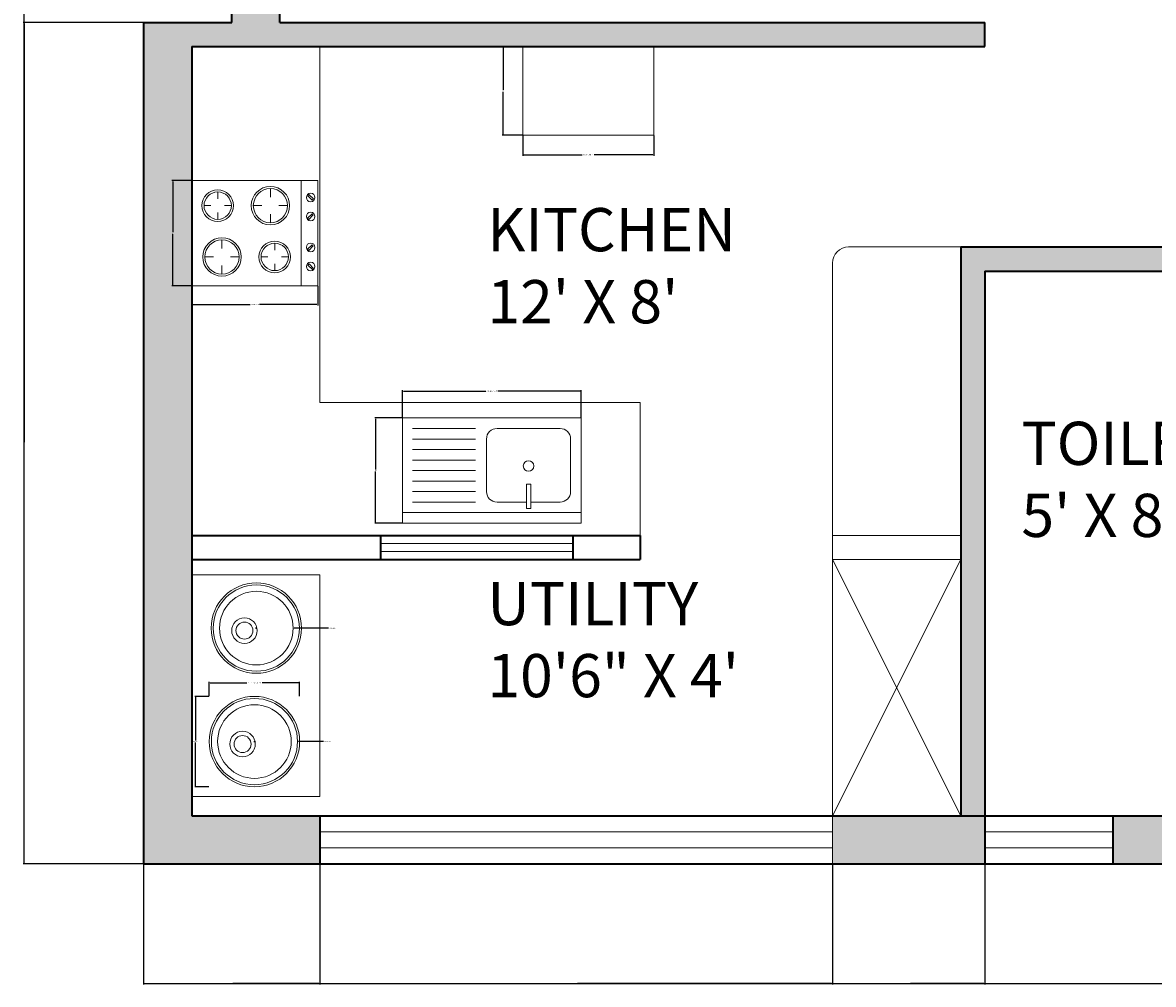
# Model space of a CAD drawing. Units: inches. Extents: x 2 to 2806, y 1095 to 1587.
# Tile 1 of 4: x 2363 to 2575, y 1095 to 1275. Entities that reach past the tile are written whole.
import ezdxf

# ---------------------------------------------------------------- set-up
doc = ezdxf.new("R2010")
doc.units = ezdxf.units.IN
for name, color, linetype, lineweight in [('A-ANNO-DIMS', 2, 'Continuous', 18), ('A-AREA-IDEN', 7, 'Continuous', 25), ('A-EQPM', 8, 'Continuous', 18), ('A-FLOR-CASE', 34, 'Continuous', 18), ('A-FLOR-FIXT', 9, 'Continuous', 18), ('A-GLAZ', 4, 'Continuous', 18), ('A-WALL', 7, 'Continuous', 35)]:
    doc.layers.add(name, color=color, linetype=linetype, lineweight=lineweight)
doc.layers.add('A-WALL-PATT', color=18, linetype='Continuous', lineweight=13, true_color=0x000000)
doc.styles.get("Standard").update_dxf_attribs({"font": 'arial.ttf'})
doc.dimstyles.get("Standard").update_dxf_attribs({"dimtxt": 0.18, "dimasz": 0.18, "dimexe": 0.18, "dimexo": 0.0625, "dimgap": 0.09, "dimtad": 0, "dimtih": 1, "dimtoh": 1, "dimdec": 4, "dimzin": 0, "dimdsep": 46, "dimtxsty": 'Standard', "dimcen": 0.09, "dimadec": 0, "dimazin": 0, "dimtfac": 1, "dimtdec": 4, "dimtofl": 0, "dimtmove": 0, "dimatfit": 3, "dimfxl": 1, "dimtolj": 1, "dimtzin": 0, "dimarcsym": 0})

# ---------------------------------------------------------------- blocks, each defined once
blk = doc.blocks.new('A$C3404121D')
for p, q in [((0, 0), (0, 500)), ((0, 500), (850, 500)), ((850, 500), (850, 0)), ((0, 450), (850, 450)), ((239.7, 430.7), (239.7, 425)), ((259.7, 430.7), (239.7, 430.7)), ((259.7, 430.7), (259.7, 315.4)), ((100, 400), (240, 400)), ((239.7, 425), (239.7, 315.4)), ((259.9, 400), (400, 400)), ((501.8, 400), (801.5, 400)), ((50, 100), (50, 350)), ((450, 100), (450, 350)), ((501.8, 350), (801.5, 350)), ((239.7, 315.4), (259.7, 315.4)), ((501.8, 300), (801.5, 300)), ((501.8, 250), (801.5, 250)), ((501.8, 200), (801.5, 200)), ((501.8, 150), (801.5, 150)), ((501.8, 100), (801.5, 100)), ((850, 0), (0, 0)), ((400, 50), (100, 50)), ((801.5, 50), (501.8, 50))]:
    blk.add_line(p, q)
blk.add_circle((250.1, 228.3), 25)
for centre, start, end in [((100, 350), 90, 180), ((400, 350), 0, 90), ((100, 100), 180, 270), ((400, 100), 270, 0)]:
    blk.add_arc(centre, 50, start, end)
blk = doc.blocks.new('A$C5A6D4E37')
for centre, radius in [((215, 215), 215), ((215, 215), 205), ((215, 215), 175), ((158.5, 203.1), 60.6), ((158.5, 203.1), 40.6)]:
    blk.add_circle(centre, radius)
blk = doc.blocks.new('A$C16A60262')
at = {"linetype": 'ByBlock'}
for p, q in [((0, 600), (0, 0)), ((487.7, 600), (0, 600)), ((0, 600), (500, 600)), ((0, 600), (500, 600)), ((500, 600), (500, 0)), ((500, 600), (500, 0)), ((500, 520.4), (0, 520.4)), ((119.4, 455.6), (119.4, 414.9)), ((363.3, 459.6), (363.3, 427.1)), ((298.2, 394.6), (330.7, 394.6)), ((428.3, 394.6), (395.8, 394.6)), ((38.1, 374.3), (78.8, 374.3)), ((119.4, 293), (119.4, 333.7)), ((200.7, 374.3), (160.1, 374.3)), ((363.3, 329.6), (363.3, 362.1)), ((363.3, 225.2), (363.3, 184.6)), ((119.4, 188.6), (119.4, 156.1)), ((54.4, 123.6), (86.9, 123.6)), ((184.4, 123.6), (151.9, 123.6)), ((282, 143.9), (322.6, 143.9)), ((444.5, 143.9), (403.9, 143.9)), ((119.4, 58.6), (119.4, 91.1)), ((363.3, 62.6), (363.3, 103.3)), ((0, 0), (500, 0))]:
    blk.add_line(p, q, dxfattribs=at)
for p, q in [((66.2, 557.5), (87.4, 578.7)), ((71.9, 551.8), (66.2, 557.5)), ((93.1, 573), (71.9, 551.8)), ((87.4, 578.7), (93.1, 573)), ((157.6, 572.5), (163.3, 578.1)), ((178.8, 551.2), (157.6, 572.5)), ((163.3, 578.1), (184.5, 556.9)), ((184.5, 556.9), (178.8, 551.2)), ((305.1, 572.5), (310.8, 578.1)), ((326.3, 551.2), (305.1, 572.5)), ((310.8, 578.1), (332, 556.9)), ((332, 556.9), (326.3, 551.2)), ((396.2, 558.5), (417.4, 579.7)), ((401.9, 552.8), (396.2, 558.5)), ((423.1, 574), (401.9, 552.8)), ((417.4, 579.7), (423.1, 574))]:
    blk.add_line(p, q)
for centre in [(80.1, 565.7), (171.2, 565.7), (317.6, 565.7), (408.7, 565.7)]:
    blk.add_circle(centre, 20.6)
for centre, radius in [((119.4, 374.3), 91.3), ((119.4, 374.3), 81.3), ((363.3, 394.6), 75), ((363.3, 394.6), 65), ((363.3, 143.9), 91.3), ((363.3, 143.9), 81.3), ((119.4, 123.6), 75), ((119.4, 123.6), 65)]:
    blk.add_circle(centre, radius, dxfattribs=at)
blk = doc.blocks.new('Group-52')
for p, q in [((0.4676, 2.032), (0.4676, 0)), ((1.8392, 2.032), (0.4676, 2.032)), ((1.8392, 0), (1.8392, 2.032)), ((0.4676, 0), (1.8392, 0))]:
    blk.add_line(p, q)
blk = doc.blocks.new('WIN-GLAZ-24x9')
for p, q in [((0, 3), (24, 3)), ((0, 0), (24, 0))]:
    blk.add_line(p, q)
blk = doc.blocks.new('*D32')
at = {"layer": 'A-ANNO-DIMS', "color": 0, "lineweight": -2, "transparency": 16777216}
for p, q in [((2397.92, 1148.65), (2397.92, 1151.31)), ((2398.1, 1151.13), (2404.95, 1151.13)), ((2414.67, 1151.13), (2407.82, 1151.13)), ((2414.85, 1148.65), (2414.85, 1151.31))]:
    blk.add_line(p, q, dxfattribs=at)
at = {"layer": 'A-ANNO-DIMS', "color": 0, "transparency": 16777216}
for points in [[(2398.1, 1151.16), (2398.1, 1151.1), (2397.92, 1151.13)], [(2414.67, 1151.16), (2414.67, 1151.1), (2414.85, 1151.13)]]:
    blk.add_solid(points, dxfattribs=at)
at = {"layer": 'Defpoints', "color": 0, "transparency": 16777216}
for p in [(2414.85, 1151.13), (2397.92, 1148.59), (2414.85, 1148.59)]:
    blk.add_point(p, dxfattribs=at)
at = {"layer": 'A-ANNO-DIMS', "color": 0, "transparency": 16777216, "insert": (2406.39, 1151.13), "char_height": 0.18, "attachment_point": 5}
blk.add_mtext('\\A1;UTILITY BASIN 17 TYP.', dxfattribs=at)
blk = doc.blocks.new('*D33')
at = {"layer": 'A-ANNO-DIMS', "color": 0, "lineweight": -2, "transparency": 16777216}
for p, q in [((2397.86, 1148.59), (2395.2, 1148.59)), ((2395.38, 1148.41), (2395.38, 1140.31)), ((2395.38, 1131.84), (2395.38, 1139.95)), ((2397.86, 1131.66), (2395.2, 1131.66))]:
    blk.add_line(p, q, dxfattribs=at)
at = {"layer": 'A-ANNO-DIMS', "color": 0, "transparency": 16777216}
for points in [[(2395.35, 1148.41), (2395.41, 1148.41), (2395.38, 1148.59)], [(2395.35, 1131.84), (2395.41, 1131.84), (2395.38, 1131.66)]]:
    blk.add_solid(points, dxfattribs=at)
at = {"layer": 'Defpoints', "color": 0, "transparency": 16777216}
for p in [(2395.38, 1148.59), (2397.92, 1148.59), (2397.92, 1131.66)]:
    blk.add_point(p, dxfattribs=at)
at = {"layer": 'A-ANNO-DIMS', "color": 0, "transparency": 16777216, "insert": (2395.38, 1140.13), "char_height": 0.18, "attachment_point": 5}
blk.add_mtext('\\A1;17 TYP.', dxfattribs=at)
blk = doc.blocks.new('*D42')
at = {"layer": 'A-ANNO-DIMS', "color": 0, "lineweight": -2, "transparency": 16777216}
for p, q in [((2434.1, 1200.77), (2434.1, 1205.9)), ((2434.28, 1205.72), (2449.7, 1205.72)), ((2467.38, 1205.72), (2451.96, 1205.72)), ((2467.56, 1200.77), (2467.56, 1205.9))]:
    blk.add_line(p, q, dxfattribs=at)
at = {"layer": 'A-ANNO-DIMS', "color": 0, "transparency": 16777216}
for points in [[(2434.28, 1205.75), (2434.28, 1205.69), (2434.1, 1205.72)], [(2467.38, 1205.75), (2467.38, 1205.69), (2467.56, 1205.72)]]:
    blk.add_solid(points, dxfattribs=at)
at = {"layer": 'Defpoints', "color": 0, "transparency": 16777216}
for p in [(2434.1, 1205.72), (2434.1, 1200.7), (2467.56, 1200.7)]:
    blk.add_point(p, dxfattribs=at)
at = {"layer": 'A-ANNO-DIMS', "color": 0, "transparency": 16777216, "insert": (2450.83, 1205.72), "char_height": 0.18, "attachment_point": 5}
blk.add_mtext('\\A1;KITCHEN SINK 33', dxfattribs=at)
blk = doc.blocks.new('*D43')
at = {"layer": 'A-ANNO-DIMS', "color": 0, "lineweight": -2, "transparency": 16777216}
for p, q in [((2434.03, 1200.7), (2428.9, 1200.7)), ((2429.08, 1200.52), (2429.08, 1191.04)), ((2429.08, 1181.2), (2429.08, 1190.68)), ((2434.03, 1181.02), (2428.9, 1181.02))]:
    blk.add_line(p, q, dxfattribs=at)
at = {"layer": 'A-ANNO-DIMS', "color": 0, "transparency": 16777216}
for points in [[(2429.05, 1200.52), (2429.11, 1200.52), (2429.08, 1200.7)], [(2429.05, 1181.2), (2429.11, 1181.2), (2429.08, 1181.02)]]:
    blk.add_solid(points, dxfattribs=at)
at = {"layer": 'Defpoints', "color": 0, "transparency": 16777216}
for p in [(2434.1, 1200.7), (2429.08, 1181.02), (2434.1, 1181.02)]:
    blk.add_point(p, dxfattribs=at)
at = {"layer": 'A-ANNO-DIMS', "color": 0, "transparency": 16777216, "insert": (2429.08, 1190.86), "char_height": 0.18, "attachment_point": 5}
blk.add_mtext('\\A1;20', dxfattribs=at)
blk = doc.blocks.new('*D44')
at = {"layer": 'A-ANNO-DIMS', "color": 0, "lineweight": -2, "transparency": 16777216}
for p, q in [((2394.64, 1225.4), (2394.64, 1221.74)), ((2418.26, 1225.4), (2418.26, 1221.74)), ((2394.82, 1221.92), (2405.57, 1221.92)), ((2418.08, 1221.92), (2407.33, 1221.92))]:
    blk.add_line(p, q, dxfattribs=at)
at = {"layer": 'A-ANNO-DIMS', "color": 0, "transparency": 16777216}
for points in [[(2394.82, 1221.95), (2394.82, 1221.89), (2394.64, 1221.92)], [(2418.08, 1221.95), (2418.08, 1221.89), (2418.26, 1221.92)]]:
    blk.add_solid(points, dxfattribs=at)
at = {"layer": 'Defpoints', "color": 0, "transparency": 16777216}
for p in [(2394.64, 1225.46), (2418.26, 1225.46), (2418.26, 1221.92)]:
    blk.add_point(p, dxfattribs=at)
at = {"layer": 'A-ANNO-DIMS', "color": 0, "transparency": 16777216, "insert": (2406.45, 1221.92), "char_height": 0.18, "attachment_point": 5}
blk.add_mtext('\\A1;COOKTOP 24', dxfattribs=at)
blk = doc.blocks.new('*D45')
at = {"layer": 'A-ANNO-DIMS', "color": 0, "lineweight": -2, "transparency": 16777216}
for p, q in [((2394.58, 1245.15), (2390.92, 1245.15)), ((2391.1, 1244.97), (2391.1, 1235.49)), ((2391.1, 1225.64), (2391.1, 1235.12)), ((2394.58, 1225.46), (2390.92, 1225.46))]:
    blk.add_line(p, q, dxfattribs=at)
at = {"layer": 'A-ANNO-DIMS', "color": 0, "transparency": 16777216}
for points in [[(2391.07, 1244.97), (2391.13, 1244.97), (2391.1, 1245.15)], [(2391.07, 1225.64), (2391.13, 1225.64), (2391.1, 1225.46)]]:
    blk.add_solid(points, dxfattribs=at)
at = {"layer": 'Defpoints', "color": 0, "transparency": 16777216}
for p in [(2394.64, 1245.15), (2391.1, 1225.46), (2394.64, 1225.46)]:
    blk.add_point(p, dxfattribs=at)
at = {"layer": 'A-ANNO-DIMS', "color": 0, "transparency": 16777216, "insert": (2391.1, 1235.31), "char_height": 0.18, "attachment_point": 5}
blk.add_mtext('\\A1;20', dxfattribs=at)
blk = doc.blocks.new('*D48')
at = {"layer": 'A-ANNO-DIMS', "color": 0, "lineweight": -2, "transparency": 16777216}
for p, q in [((2456.62, 1253.58), (2456.62, 1249.78)), ((2481.17, 1253.58), (2481.17, 1249.78)), ((2456.8, 1249.96), (2467.76, 1249.96)), ((2480.99, 1249.96), (2470.02, 1249.96))]:
    blk.add_line(p, q, dxfattribs=at)
at = {"layer": 'A-ANNO-DIMS', "color": 0, "transparency": 16777216}
for points in [[(2456.8, 1249.99), (2456.8, 1249.93), (2456.62, 1249.96)], [(2480.99, 1249.99), (2480.99, 1249.93), (2481.17, 1249.96)]]:
    blk.add_solid(points, dxfattribs=at)
at = {"layer": 'Defpoints', "color": 0, "transparency": 16777216}
for p in [(2456.62, 1253.64), (2481.17, 1253.64), (2481.17, 1249.96)]:
    blk.add_point(p, dxfattribs=at)
at = {"layer": 'A-ANNO-DIMS', "color": 0, "transparency": 16777216, "insert": (2468.89, 1249.96), "char_height": 0.18, "attachment_point": 5}
blk.add_mtext('\\A1;KITCHEN UNIT 25', dxfattribs=at)
blk = doc.blocks.new('*D49')
at = {"layer": 'A-ANNO-DIMS', "color": 0, "lineweight": -2, "transparency": 16777216}
for p, q in [((2456.55, 1270.21), (2452.75, 1270.21)), ((2452.93, 1270.03), (2452.93, 1262.11)), ((2452.93, 1253.82), (2452.93, 1261.75)), ((2456.55, 1253.64), (2452.75, 1253.64))]:
    blk.add_line(p, q, dxfattribs=at)
at = {"layer": 'A-ANNO-DIMS', "color": 0, "transparency": 16777216}
for points in [[(2452.9, 1270.03), (2452.96, 1270.03), (2452.93, 1270.21)], [(2452.9, 1253.82), (2452.96, 1253.82), (2452.93, 1253.64)]]:
    blk.add_solid(points, dxfattribs=at)
at = {"layer": 'Defpoints', "color": 0, "transparency": 16777216}
for p in [(2456.62, 1270.21), (2452.93, 1253.64), (2456.62, 1253.64)]:
    blk.add_point(p, dxfattribs=at)
at = {"layer": 'A-ANNO-DIMS', "color": 0, "transparency": 16777216, "insert": (2452.93, 1261.93), "char_height": 0.18, "attachment_point": 5}
blk.add_mtext('\\A1;17', dxfattribs=at)
blk = doc.blocks.new('*D54')
at = {"layer": 'A-ANNO-DIMS', "color": 0, "lineweight": -2, "transparency": 16777216}
for p, q in [((2385.64, 1117.15), (2385.64, 1094.67)), ((2783.14, 1117.15), (2783.14, 1094.67)), ((2385.82, 1094.85), (2584, 1094.85)), ((2782.96, 1094.85), (2584.79, 1094.85))]:
    blk.add_line(p, q, dxfattribs=at)
at = {"layer": 'A-ANNO-DIMS', "color": 0, "transparency": 16777216}
for points in [[(2385.82, 1094.88), (2385.82, 1094.82), (2385.64, 1094.85)], [(2782.96, 1094.88), (2782.96, 1094.82), (2783.14, 1094.85)]]:
    blk.add_solid(points, dxfattribs=at)
at = {"layer": 'Defpoints', "color": 0, "transparency": 16777216}
for p in [(2385.64, 1117.21), (2783.14, 1117.21), (2783.14, 1094.85)]:
    blk.add_point(p, dxfattribs=at)
at = {"layer": 'A-ANNO-DIMS', "color": 0, "transparency": 16777216, "insert": (2584.39, 1094.85), "char_height": 0.18, "attachment_point": 5}
blk.add_mtext('\\A1;397.5', dxfattribs=at)
blk = doc.blocks.new('*D57')
at = {"layer": 'A-ANNO-DIMS', "color": 0, "lineweight": -2, "transparency": 16777216}
for p, q in [((2385.580192, 1564.213452), (2363.102692, 1564.213452)), ((2363.282692, 1564.033452), (2363.282692, 1340.893452)), ((2363.282692, 1117.393452), (2363.282692, 1340.533452)), ((2385.580192, 1117.213452), (2363.102692, 1117.213452))]:
    blk.add_line(p, q, dxfattribs=at)
at = {"layer": 'A-ANNO-DIMS', "color": 0, "transparency": 16777216}
for points in [[(2363.252692, 1564.033452), (2363.312692, 1564.033452), (2363.282692, 1564.213452)], [(2363.252692, 1117.393452), (2363.312692, 1117.393452), (2363.282692, 1117.213452)]]:
    blk.add_solid(points, dxfattribs=at)
at = {"layer": 'Defpoints', "color": 0, "transparency": 16777216}
for p in [(2363.282692, 1564.213452), (2385.642692, 1564.213452), (2385.642692, 1117.213452)]:
    blk.add_point(p, dxfattribs=at)
at = {"layer": 'A-ANNO-DIMS', "color": 0, "transparency": 16777216, "insert": (2363.282692, 1340.713452), "char_height": 0.18, "attachment_point": 5}
blk.add_mtext('\\A1;447', dxfattribs=at)
blk = doc.blocks.new('*D67')
at = {"layer": 'A-ANNO-DIMS', "color": 0, "lineweight": -2, "transparency": 16777216}
for p, q in [((2385.64, 1117.15), (2385.64, 1094.67)), ((2418.64, 1117.15), (2418.64, 1094.67)), ((2385.82, 1094.85), (2401.92, 1094.85)), ((2418.46, 1094.85), (2402.36, 1094.85))]:
    blk.add_line(p, q, dxfattribs=at)
at = {"layer": 'A-ANNO-DIMS', "color": 0, "transparency": 16777216}
for points in [[(2385.82, 1094.88), (2385.82, 1094.82), (2385.64, 1094.85)], [(2418.46, 1094.88), (2418.46, 1094.82), (2418.64, 1094.85)]]:
    blk.add_solid(points, dxfattribs=at)
at = {"layer": 'Defpoints', "color": 0, "transparency": 16777216}
for p in [(2385.64, 1117.21), (2418.64, 1117.21), (2418.64, 1094.85)]:
    blk.add_point(p, dxfattribs=at)
at = {"layer": 'A-ANNO-DIMS', "color": 0, "transparency": 16777216, "insert": (2402.14, 1094.85), "char_height": 0.18, "attachment_point": 5}
blk.add_mtext('\\A1;33', dxfattribs=at)
blk = doc.blocks.new('*D68')
at = {"layer": 'A-ANNO-DIMS', "color": 0, "lineweight": -2, "transparency": 16777216}
for p, q in [((2418.64, 1117.15), (2418.64, 1094.67)), ((2514.64, 1117.15), (2514.64, 1094.67)), ((2418.82, 1094.85), (2466.42, 1094.85)), ((2514.46, 1094.85), (2466.86, 1094.85))]:
    blk.add_line(p, q, dxfattribs=at)
at = {"layer": 'A-ANNO-DIMS', "color": 0, "transparency": 16777216}
for points in [[(2418.82, 1094.88), (2418.82, 1094.82), (2418.64, 1094.85)], [(2514.46, 1094.88), (2514.46, 1094.82), (2514.64, 1094.85)]]:
    blk.add_solid(points, dxfattribs=at)
at = {"layer": 'Defpoints', "color": 0, "transparency": 16777216}
for p in [(2418.64, 1117.21), (2514.64, 1117.21), (2514.64, 1094.85)]:
    blk.add_point(p, dxfattribs=at)
at = {"layer": 'A-ANNO-DIMS', "color": 0, "transparency": 16777216, "insert": (2466.64, 1094.85), "char_height": 0.18, "attachment_point": 5}
blk.add_mtext('\\A1;96', dxfattribs=at)
blk = doc.blocks.new('*D69')
at = {"layer": 'A-ANNO-DIMS', "color": 0, "lineweight": -2, "transparency": 16777216}
for p, q in [((2514.64, 1117.15), (2514.64, 1094.67)), ((2543.14, 1117.15), (2543.14, 1094.67)), ((2514.82, 1094.85), (2528.57, 1094.85)), ((2542.96, 1094.85), (2529.22, 1094.85))]:
    blk.add_line(p, q, dxfattribs=at)
at = {"layer": 'A-ANNO-DIMS', "color": 0, "transparency": 16777216}
for points in [[(2514.82, 1094.88), (2514.82, 1094.82), (2514.64, 1094.85)], [(2542.96, 1094.88), (2542.96, 1094.82), (2543.14, 1094.85)]]:
    blk.add_solid(points, dxfattribs=at)
at = {"layer": 'Defpoints', "color": 0, "transparency": 16777216}
for p in [(2514.64, 1117.21), (2543.14, 1117.21), (2543.14, 1094.85)]:
    blk.add_point(p, dxfattribs=at)
at = {"layer": 'A-ANNO-DIMS', "color": 0, "transparency": 16777216, "insert": (2528.89, 1094.85), "char_height": 0.18, "attachment_point": 5}
blk.add_mtext('\\A1;28.5', dxfattribs=at)
blk = doc.blocks.new('*D72')
at = {"layer": 'A-ANNO-DIMS', "color": 0, "lineweight": -2, "transparency": 16777216}
for p, q in [((2385.58, 1274.71), (2363.1, 1274.71)), ((2363.28, 1274.53), (2363.28, 1196.15)), ((2363.28, 1117.39), (2363.28, 1195.78)), ((2385.58, 1117.21), (2363.1, 1117.21))]:
    blk.add_line(p, q, dxfattribs=at)
at = {"layer": 'A-ANNO-DIMS', "color": 0, "transparency": 16777216}
for points in [[(2363.25, 1274.53), (2363.31, 1274.53), (2363.28, 1274.71)], [(2363.25, 1117.39), (2363.31, 1117.39), (2363.28, 1117.21)]]:
    blk.add_solid(points, dxfattribs=at)
at = {"layer": 'Defpoints', "color": 0, "transparency": 16777216}
for p in [(2363.28, 1274.71), (2385.64, 1274.71), (2385.64, 1117.21)]:
    blk.add_point(p, dxfattribs=at)
at = {"layer": 'A-ANNO-DIMS', "color": 0, "transparency": 16777216, "insert": (2363.28, 1195.96), "char_height": 0.18, "attachment_point": 5}
blk.add_mtext('\\A1;157.5', dxfattribs=at)
blk = doc.blocks.new('*D79')
at = {"layer": 'A-ANNO-DIMS', "color": 0, "lineweight": -2, "transparency": 16777216}
for p, q in [((2406.65, 1161.37), (2406.83, 1161.37)), ((2406.74, 1161.28), (2406.74, 1161.46)), ((2420.28, 1161.37), (2415.38, 1161.37))]:
    blk.add_line(p, q, dxfattribs=at)
at = {"layer": 'A-ANNO-DIMS', "color": 0, "transparency": 16777216}
blk.add_solid([(2415.38, 1161.4), (2415.38, 1161.34), (2415.2, 1161.37)], dxfattribs=at)
at = {"layer": 'Defpoints', "color": 0, "transparency": 16777216}
for p in [(2398.28, 1161.37), (2415.2, 1161.37)]:
    blk.add_point(p, dxfattribs=at)
at = {"layer": 'A-ANNO-DIMS', "color": 0, "transparency": 16777216, "insert": (2420.97, 1161.37), "char_height": 0.18, "attachment_point": 5}
blk.add_mtext('\\A1;2X ∅16.93', dxfattribs=at)
blk = doc.blocks.new('*D80')
at = {"layer": 'A-ANNO-DIMS', "color": 0, "lineweight": -2, "transparency": 16777216}
for p, q in [((2406.3, 1140.13), (2406.48, 1140.13)), ((2406.39, 1140.04), (2406.39, 1140.22)), ((2419.3, 1140.13), (2414.64, 1140.13))]:
    blk.add_line(p, q, dxfattribs=at)
at = {"layer": 'A-ANNO-DIMS', "color": 0, "transparency": 16777216}
blk.add_solid([(2414.64, 1140.16), (2414.64, 1140.1), (2414.46, 1140.13)], dxfattribs=at)
at = {"layer": 'Defpoints', "color": 0, "transparency": 16777216}
for p in [(2398.31, 1140.13), (2414.46, 1140.13)]:
    blk.add_point(p, dxfattribs=at)
at = {"layer": 'A-ANNO-DIMS', "color": 0, "transparency": 16777216, "insert": (2420.05, 1140.13), "char_height": 0.18, "attachment_point": 5}
blk.add_mtext('\\A1;2X ∅16.142', dxfattribs=at)
blk = doc.blocks.new('*D81')
at = {"layer": 'A-ANNO-DIMS', "color": 0, "lineweight": -2, "transparency": 16777216}
for p, q in [((2406.65, 1161.37), (2406.83, 1161.37)), ((2406.74, 1161.28), (2406.74, 1161.46)), ((2417.76, 1161.37), (2413.81, 1161.37))]:
    blk.add_line(p, q, dxfattribs=at)
at = {"layer": 'A-ANNO-DIMS', "color": 0, "transparency": 16777216}
blk.add_solid([(2413.81, 1161.4), (2413.81, 1161.34), (2413.63, 1161.37)], dxfattribs=at)
at = {"layer": 'Defpoints', "color": 0, "transparency": 16777216}
for p in [(2399.85, 1161.37), (2413.63, 1161.37)]:
    blk.add_point(p, dxfattribs=at)
at = {"layer": 'A-ANNO-DIMS', "color": 0, "transparency": 16777216, "insert": (2418.45, 1161.37), "char_height": 0.18, "attachment_point": 5}
blk.add_mtext('\\A1;2X ∅13.78', dxfattribs=at)

msp = doc.modelspace()

# ---------------------------------------------------------------- hatches: boundary and pattern name
at = {"layer": 'A-WALL-PATT'}
h = msp.add_hatch(color=256, dxfattribs=at)
h.dxf.hatch_style = 1
h.paths.add_polyline_path([(2444, 1564.2135), (2385.6427, 1564.2135), (2385.6427, 1465.2135), (2394.6427, 1465.2135), (2394.6427, 1555.2135), (2444, 1555.2135)])
h.paths.add_polyline_path([(2540, 1564.2135), (2480, 1564.2135), (2480, 1555.2135), (2514.6427, 1555.2135), (2514.6427, 1448.7135), (2550.1001, 1448.7135), (2550.1001, 1453.2135), (2519.1427, 1453.2135), (2519.1427, 1555.2135), (2540, 1555.2135)])
h.paths.add_polyline_path([(2619.6427, 1564.2135), (2564, 1564.2135), (2564, 1555.2135), (2579.1427, 1555.2135), (2579.1427, 1453.2135), (2577.7846, 1453.2135), (2577.7846, 1448.7135), (2648.1427, 1448.7135), (2648.1427, 1497.3535), (2643.6427, 1497.3535), (2643.6427, 1453.2135), (2583.6427, 1453.2135), (2583.6427, 1555.2135), (2619.6427, 1555.2135)])
h.paths.add_polyline_path([(2658, 1564.2135), (2643.6427, 1564.2135), (2643.6427, 1555.2135), (2643.6427, 1521.3535), (2648.1427, 1521.3535), (2648.1427, 1555.2135), (2658, 1555.2135)])
h.paths.add_polyline_path([(2783.1427, 1564.2135), (2730, 1564.2135), (2730, 1555.2135), (2774.1427, 1555.2135), (2774.1427, 1465.3633), (2783.1427, 1465.3633)])
h.paths.add_polyline_path([(2783.1427, 1429.3633), (2774.1427, 1429.3633), (2774.1427, 1411.2135), (2610.5887, 1411.2135), (2610.5887, 1406.7135), (2774.1427, 1406.7135), (2774.1427, 1394.7135), (2783.1427, 1394.7135)])
h.paths.add_polyline_path([(2783.1427, 1358.7135), (2774.1427, 1358.7135), (2774.1427, 1336), (2783.1427, 1336)])
h.paths.add_polyline_path([(2783.1427, 1300), (2774.1427, 1300), (2774.1427, 1274.7135), (2646.5887, 1274.7135), (2646.5887, 1270.2135), (2774.1427, 1270.2135), (2774.1427, 1126.2135), (2750.1427, 1126.2135), (2750.1427, 1117.2135), (2783.1427, 1117.2135)])
h.paths.add_polyline_path([(2607.6427, 1126.2135), (2567.1427, 1126.2135), (2567.1427, 1117.2135), (2607.6427, 1117.2135)])
h.paths.add_polyline_path([(2714.1427, 1126.2135), (2643.6427, 1126.2135), (2643.6427, 1117.2135), (2714.1427, 1117.2135)])
h.paths.add_polyline_path([(2607.6427, 1270.2135), (2610.5887, 1270.2135), (2610.5887, 1274.7135), (2579.1427, 1274.7135), (2579.1427, 1270.2135), (2603.1427, 1270.2135), (2603.1427, 1232.7135), (2538.6427, 1232.7135), (2538.6427, 1126.2135), (2543.1427, 1126.2135), (2543.1427, 1228.2135), (2603.1427, 1228.2135), (2603.1427, 1189.2001), (2607.6427, 1189.2001)])
h.paths.add_polyline_path([(2543.1427, 1126.2135), (2514.6427, 1126.2135), (2514.6427, 1117.2135), (2543.1427, 1117.2135)], flags=17)
h.paths.add_polyline_path([(2418.6427, 1126.2135), (2394.6427, 1126.2135), (2394.6427, 1270.2135), (2418.6427, 1270.2135), (2543.1427, 1270.2135), (2543.1427, 1274.7135), (2411.1427, 1274.7135), (2411.1427, 1310), (2402.1427, 1310), (2402.1427, 1274.7135), (2385.6427, 1274.7135), (2385.6427, 1117.2135), (2418.6427, 1117.2135)])
h.paths.add_polyline_path([(2543.1427, 1411.2135), (2394.6427, 1411.2135), (2394.6427, 1429.2135), (2385.6427, 1429.2135), (2385.6427, 1406.7135), (2402.1427, 1406.7135), (2402.1427, 1370), (2411.1427, 1370), (2411.1427, 1406.7135), (2543.1427, 1406.7135)])

# ---------------------------------------------------------------- linework, layer by layer
at = {"layer": 'A-FLOR-CASE'}
for p, q in [((2394.6427, 1270.2135), (2418.6427, 1270.2135)), ((2418.6427, 1270.2135), (2418.6427, 1203.5997)), ((2538.6427, 1232.7135), (2517.6427, 1232.7135)), ((2514.6427, 1229.7135), (2514.6427, 1117.2135)), ((2418.6427, 1203.5997), (2478.6427, 1203.5997)), ((2478.6427, 1203.5997), (2478.6427, 1178.7135)), ((2514.6427, 1178.7135), (2538.6427, 1178.7135)), ((2514.6427, 1174.2135), (2538.6427, 1174.2135)), ((2514.6427, 1174.2135), (2538.6427, 1126.2135)), ((2538.6427, 1174.2135), (2514.6427, 1126.2135)), ((2418.6427, 1171.3236), (2394.6427, 1171.3236)), ((2418.6427, 1171.3236), (2418.6427, 1129.8376)), ((2394.6427, 1129.8376), (2418.6427, 1129.8376))]:
    msp.add_line(p, q, dxfattribs=at)
msp.add_arc((2517.6427, 1229.7135), 3, 90, 180, dxfattribs=at)
at = {"layer": 'A-GLAZ'}
for p, q in [((2430, 1177.2135), (2466, 1177.2135)), ((2430, 1175.7135), (2466, 1175.7135)), ((2418.6427, 1123.2135), (2514.6427, 1123.2135)), ((2418.6427, 1120.2135), (2514.6427, 1120.2135))]:
    msp.add_line(p, q, dxfattribs=at)
at = {"layer": 'A-WALL'}
for p, q in [((2402.1427, 1274.7135), (2402.1427, 1406.7135)), ((2411.1427, 1274.7135), (2411.1427, 1406.7135)), ((2385.6427, 1274.7135), (2402.1427, 1274.7135)), ((2385.6427, 1274.7135), (2385.6427, 1117.2135)), ((2411.1427, 1274.7135), (2543.1427, 1274.7135)), ((2543.1427, 1270.2135), (2543.1427, 1274.7135)), ((2394.6427, 1270.2135), (2543.1427, 1270.2135)), ((2394.6427, 1270.2135), (2394.6427, 1126.2135)), ((2538.6427, 1232.7135), (2538.6427, 1126.2135)), ((2538.6427, 1232.7135), (2603.1427, 1232.7135)), ((2543.1427, 1228.2135), (2603.1427, 1228.2135)), ((2543.1427, 1228.2135), (2543.1427, 1126.2135)), ((2394.6427, 1178.7135), (2478.6427, 1178.7135)), ((2430, 1178.7135), (2430, 1174.2135)), ((2466, 1178.7135), (2466, 1174.2135)), ((2478.6427, 1178.7135), (2478.6427, 1174.2135)), ((2394.6427, 1174.2135), (2478.6427, 1174.2135)), ((2394.6427, 1126.2135), (2774.1427, 1126.2135)), ((2418.6427, 1126.2135), (2418.6427, 1117.2135)), ((2543.1427, 1126.2135), (2543.1427, 1117.2135)), ((2567.1427, 1126.2135), (2567.1427, 1117.2135)), ((2385.6427, 1117.2135), (2783.1427, 1117.2135))]:
    msp.add_line(p, q, dxfattribs=at)

# ---------------------------------------------------------------- block references
at = {"layer": 'A-EQPM', "rotation": 270}
for name, p, xscale, yscale, zscale in [('Group-52', (2456.6162, 1275.8635), 12.08317631045745, 12.08317631045745, 12.08317631045745), ('A$C16A60262', (2394.6427, 1245.1489), 0.0393700787401575, 0.0393700787401575, 0.0393700787401575)]:
    msp.add_blockref(name, p, dxfattribs=dict(at, xscale=xscale, yscale=yscale, zscale=zscale))
at = {"layer": 'A-FLOR-FIXT', "xscale": 0.0393700787401575, "yscale": 0.0393700787401575, "zscale": 0.0393700787401575, "rotation": 180}
msp.add_blockref('A$C3404121D', (2467.5596, 1200.7033), dxfattribs=at)
at = {"layer": 'A-FLOR-FIXT', "xscale": 0.0393700787401575, "yscale": 0.0393700787401575, "zscale": 0.0393700787401575}
for p in [(2398.2754, 1152.9025), (2397.9212, 1131.6628)]:
    msp.add_blockref('A$C5A6D4E37', p, dxfattribs=at)
at = {"layer": 'A-GLAZ'}
msp.add_blockref('WIN-GLAZ-24x9', (2543.1427, 1120.2135), dxfattribs=at)

# ---------------------------------------------------------------- texts
at = {"layer": 'A-AREA-IDEN', "insert": (2450, 1240), "char_height": 8.08939, "width": 77.292105, "attachment_point": 1}
msp.add_mtext("KITCHEN\\P12' X 8'", dxfattribs=at)
at = {"layer": 'A-AREA-IDEN', "char_height": 8.08939, "attachment_point": 1}
for s, insert in [('TOILET\\P5\' X 8\'6"', (2550, 1200)), ('UTILITY\\P10\'6" X 4\'', (2450, 1170))]:
    msp.add_mtext(s, dxfattribs=dict(at, insert=insert))

# ---------------------------------------------------------------- dimensions: what is measured, and where the dimension line sits
at = {"layer": 'A-ANNO-DIMS'}
for base, p1, p2, angle, override, picture, middle in [((2363.2827, 1564.2135), (2385.6427, 1117.2135), (2385.6427, 1564.2135), 90, {"dimdec": 0, "dimlfac": 1, "dimrnd": 0, "dimzin": 0, "dimdsep": 46, "dimlunit": 2}, '*D57', (2363.2827, 1340.7135)), ((2363.2827, 1274.7135), (2385.6427, 1117.2135), (2385.6427, 1274.7135), 90, {"dimdec": 1, "dimlfac": 1, "dimrnd": 0, "dimzin": 0, "dimdsep": 46, "dimlunit": 2}, '*D72', (2363.2827, 1195.9635)), ((2452.9332, 1253.6402), (2456.6162, 1270.2135), (2456.6162, 1253.6402), 270, {"dimdec": 0, "dimlfac": 1, "dimrnd": 0, "dimzin": 0, "dimdsep": 46, "dimlunit": 2}, '*D49', (2452.9332, 1261.9268)), ((2391.0994, 1225.4638), (2394.6427, 1245.1489), (2394.6427, 1225.4638), 270, {"dimdec": 0, "dimlfac": 1, "dimrnd": 0, "dimzin": 0, "dimdsep": 46, "dimlunit": 2}, '*D45', (2391.0994, 1235.3063)), ((2429.0754, 1181.0183), (2434.0951, 1200.7033), (2434.0951, 1181.0183), 270, {"dimdec": 0, "dimlfac": 1, "dimrnd": 0, "dimzin": 0, "dimdsep": 46, "dimlunit": 2}, '*D43', (2429.0754, 1190.8608))]:
    dim = msp.add_linear_dim(base=base, p1=p1, p2=p2, angle=angle, dimstyle='Standard', override=override, dxfattribs=at)
    dim.commit()
    dim.dimension.update_dxf_attribs({"geometry": picture, "text_midpoint": middle})
for base, p1, p2, text, picture, middle in [((2481.1692, 1249.9572), (2456.6162, 1253.6402), (2481.1692, 1253.6402), 'KITCHEN UNIT <>', '*D48', (2468.8927, 1249.9572)), ((2418.2647, 1221.9205), (2394.6427, 1225.4638), (2418.2647, 1225.4638), 'COOKTOP <>', '*D44', (2406.4537, 1221.9205)), ((2414.8503, 1151.1313), (2397.9212, 1148.5919), (2414.8503, 1148.5919), 'UTILITY BASIN <> TYP.', '*D32', (2406.3857, 1151.1313))]:
    dim = msp.add_linear_dim(base=base, p1=p1, p2=p2, text=text, dimstyle='Standard', override={"dimdec": 0, "dimlfac": 1, "dimrnd": 0, "dimzin": 0, "dimdsep": 46, "dimlunit": 2}, dxfattribs=at)
    dim.commit()
    dim.dimension.update_dxf_attribs({"geometry": picture, "text_midpoint": middle})
for base, p1, p2, angle, text, picture, middle in [((2434.0951, 1205.723), (2467.5596, 1200.7033), (2434.0951, 1200.7033), 180, 'KITCHEN SINK <>', '*D42', (2450.8274, 1205.723)), ((2395.3818, 1148.5919), (2397.9212, 1131.6628), (2397.9212, 1148.5919), 90, '<> TYP.', '*D33', (2395.3818, 1140.1273))]:
    dim = msp.add_linear_dim(base=base, p1=p1, p2=p2, angle=angle, text=text, dimstyle='Standard', override={"dimdec": 0, "dimlfac": 1, "dimrnd": 0, "dimzin": 0, "dimdsep": 46, "dimlunit": 2}, dxfattribs=at)
    dim.commit()
    dim.dimension.update_dxf_attribs({"geometry": picture, "text_midpoint": middle})
for p1, p2, override, picture, middle in [((2398.2754, 1161.3671), (2415.2046, 1161.367), {"dimdec": 2, "dimlfac": 1, "dimrnd": 0, "dimzin": 0, "dimdsep": 46, "dimlunit": 2}, '*D79', (2420.2833, 1161.367)), ((2399.8502, 1161.3671), (2413.6298, 1161.367), {"dimdec": 2, "dimlfac": 1, "dimrnd": 0, "dimzin": 0, "dimdsep": 46, "dimlunit": 2}, '*D81', (2417.7636, 1161.367)), ((2398.3149, 1140.1277), (2414.4566, 1140.127), {"dimdec": 3, "dimlfac": 1, "dimrnd": 0, "dimzin": 0, "dimdsep": 46, "dimlunit": 2}, '*D80', (2419.2991, 1140.1268))]:
    dim = msp.add_diameter_dim_2p(p1=p1, p2=p2, text='2X <>', dimstyle='Standard', override=override, dxfattribs=at)
    dim.commit()
    dim.dimension.update_dxf_attribs({"geometry": picture, "text_midpoint": middle, "dimtype": 163})
for base, p1, p2, override, picture, middle in [((2783.1427, 1094.8535), (2385.6427, 1117.2135), (2783.1427, 1117.2135), {"dimdec": 1, "dimlfac": 1, "dimrnd": 0, "dimzin": 0, "dimdsep": 46, "dimlunit": 2}, '*D54', (2584.3927, 1094.8535)), ((2418.6427, 1094.8535), (2385.6427, 1117.2135), (2418.6427, 1117.2135), {"dimdec": 0, "dimlfac": 1, "dimrnd": 0, "dimzin": 0, "dimdsep": 46, "dimlunit": 2}, '*D67', (2402.1427, 1094.8535)), ((2514.6427, 1094.8535), (2418.6427, 1117.2135), (2514.6427, 1117.2135), {"dimdec": 0, "dimlfac": 1, "dimrnd": 0, "dimzin": 0, "dimdsep": 46, "dimlunit": 2}, '*D68', (2466.6427, 1094.8535)), ((2543.1427, 1094.8535), (2514.6427, 1117.2135), (2543.1427, 1117.2135), {"dimdec": 1, "dimlfac": 1, "dimrnd": 0, "dimzin": 0, "dimdsep": 46, "dimlunit": 2}, '*D69', (2528.8927, 1094.8535))]:
    dim = msp.add_linear_dim(base=base, p1=p1, p2=p2, dimstyle='Standard', override=override, dxfattribs=at)
    dim.commit()
    dim.dimension.update_dxf_attribs({"geometry": picture, "text_midpoint": middle})

doc.saveas('drawing.dxf')
